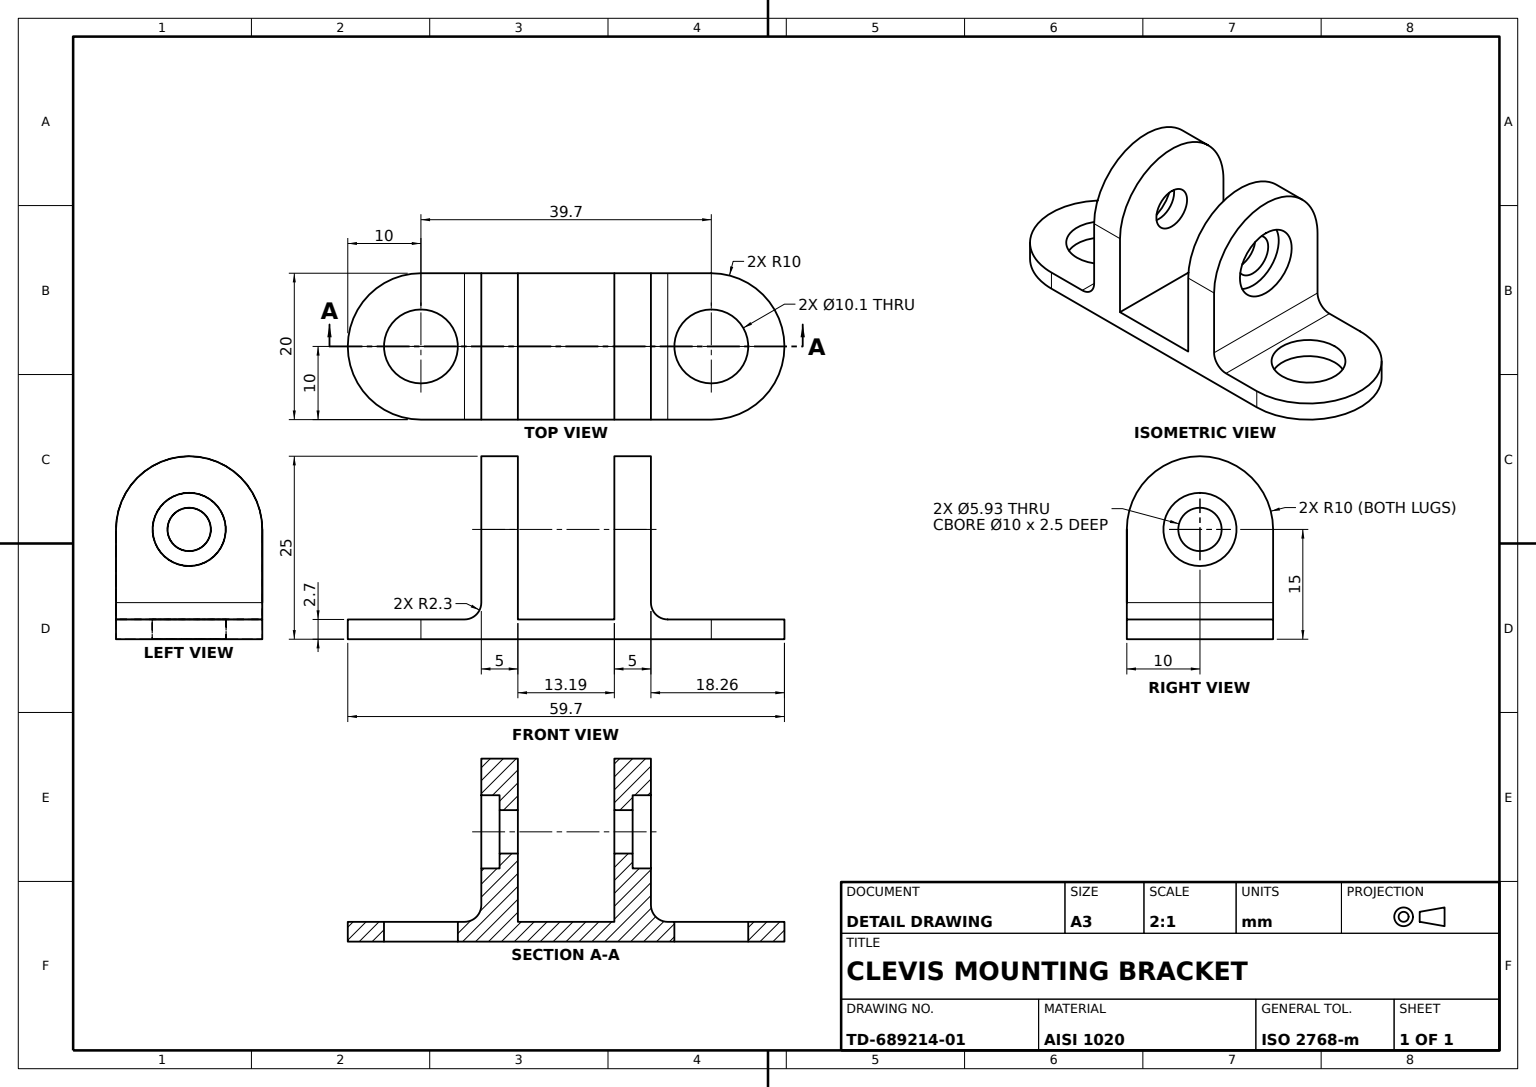
from build123d import *

# Parameters (mm, degrees)
BASE_PLATE_SKETCH_R      = 5.05
BASE_PLATE_DEPTH         = 2.7
LUG_SKETCH_W             = 5
LUG_SKETCH_H             = 12.3
LUG_DEPTH                = 20
LUG_WEB_DEPTH            = 5
FILLET_R2_3_R            = 2.3
PIN_HOLE_SKETCH_R        = 2.965
PIN_HOLE_5_93_DEPTH      = 5
COUNTERBORE_SKETCH_R     = 5
COUNTERBORE_10X2_5_DEPTH = 2.5


with BuildPart() as part:
    # Base Plate Sketch → Base Plate (new body)
    with BuildSketch(Plane(origin=(0, 0, 0), x_dir=(1, 0, 0), z_dir=(0, 1, 0))):
        with BuildLine():
            Line((-19.85, 10), (19.85, 10))
            ThreePointArc((19.85, 10), (29.85, 0), (19.85, -10))
            Line((19.85, -10), (-19.85, -10))
            ThreePointArc((-19.85, -10), (-29.85, 0), (-19.85, 10))
        make_face()
        with Locations(Location((-19.85, 0, 0), (0, 0, 90))):
            Circle(BASE_PLATE_SKETCH_R, mode=Mode.SUBTRACT)
        with Locations(Location((19.85, 0, 0), (0, 0, 90))):
            Circle(BASE_PLATE_SKETCH_R, mode=Mode.SUBTRACT)
    extrude(amount=BASE_PLATE_DEPTH)

    # Lug Sketch → Lug (add)
    with BuildSketch(Plane.XY.offset(10)):
        with Locations((-9.095, 8.85)):
            Rectangle(LUG_SKETCH_W, LUG_SKETCH_H)
    extrude(amount=-LUG_DEPTH)

    # Lug Web Sketch → Lug Web (add)
    with BuildSketch(Plane.ZY.offset(11.595)):
        with BuildLine():
            Line((-10, 15), (10, 15))
            ThreePointArc((10, 15), (0, 25), (-10, 15))
        make_face()
    extrude(amount=-LUG_WEB_DEPTH)

    # Base Plate Mirror: part across plane


with BuildPart() as part_1:
    add(part.part)
    add(part.part.mirror(Plane(origin=(0, 0, 0), x_dir=(0, 0, 1), z_dir=(1, 0, 0))))

    # Fillet R2.3
    fillet_r2_3_edges = [part_1.edges().sort_by_distance(p)[0] for p in [
        (-11.595, 2.7, 0),
        (11.595, 2.7, 0),
    ]]
    fillet(fillet_r2_3_edges, radius=FILLET_R2_3_R)

    # Pin Hole Sketch → Pin Hole Ø5.93 (cut)
    with BuildSketch(Plane.ZY.offset(11.595)):
        with Locations(Location((0, 15, 0), (0, 0, 270))):
            Circle(PIN_HOLE_SKETCH_R)
    pin_hole_5_93 = extrude(amount=-PIN_HOLE_5_93_DEPTH, mode=Mode.SUBTRACT)

    # Counterbore Sketch → Counterbore Ø10x2.5 (cut)
    with BuildSketch(Plane.ZY.offset(11.595)):
        with Locations(Location((0, 15, 0), (0, 0, 270))):
            Circle(COUNTERBORE_SKETCH_R)
    counterbore_10x2_5 = extrude(amount=-COUNTERBORE_10X2_5_DEPTH, mode=Mode.SUBTRACT)

    # Pin Hole Mirror: Pin Hole Ø5.93, Counterbore Ø10x2.5 across plane
    add(pin_hole_5_93.mirror(Plane(origin=(0, 0, 0), x_dir=(0, 0, 1), z_dir=(1, 0, 0))), mode=Mode.SUBTRACT)
    add(counterbore_10x2_5.mirror(Plane(origin=(0, 0, 0), x_dir=(0, 0, 1), z_dir=(1, 0, 0))), mode=Mode.SUBTRACT)


solid = part_1.part
